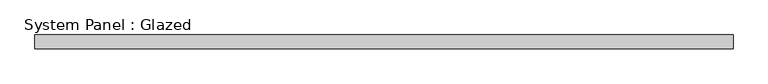
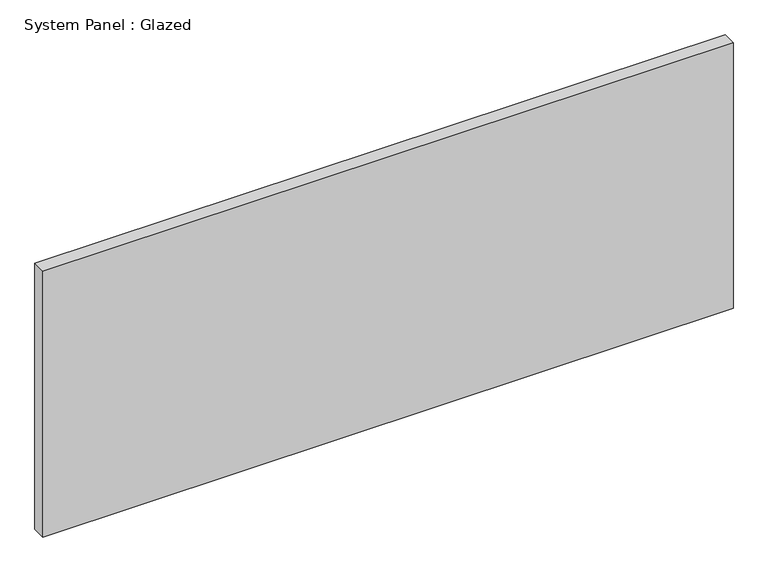
"""IFC4 building model written with IfcOpenShell, lengths in millimetres: plate geometry, System Panel : Glazed."""

from ifc_helpers import new_model, si_unit, origin, origin_with_axes, place, context, project, spatial, polyline, outline, extrude, source, transform, mapped, element, save


def system_panel_glazed_82b35773(model_context):
    return source(origin(), model_context, "Body", "SweptSolid", [
        extrude(outline(polyline([(632.0323546, 19.05), (-632.0323546, 19.05), (-632.0323546, 44.45), (632.0323546, 44.45), (632.0323546, 19.05)])), origin_with_axes(), (0.0, 0.0, 1.0), 514.35),
    ])


if __name__ == "__main__":
    model = new_model("IFC4")
    model_context = context("Model", 3, world=origin())
    ifc_project = project(units=[si_unit("LENGTHUNIT", "METRE", prefix="MILLI")], contexts=[model_context])
    site = spatial("IfcSite", under=ifc_project)
    building = spatial("IfcBuilding", under=site)
    placement = place(None, origin())
    system_panel_glazed_shape = system_panel_glazed_82b35773(model_context)
    element("IfcPlate", 1, ObjectType="System Panel : Glazed", at=placement, inside=building, context=model_context, shape_type="MappedRepresentation", body=[
        mapped(system_panel_glazed_shape, transform((0.0, 0.0, 0.0), x_axis=(1.0, 0.0, 0.0), y_axis=(0.0, 1.0, 0.0), z_axis=(0.0, 0.0, 1.0))),
    ])
    save(model, "model.ifc")

# Revit data of these elements
# Type "System Panel : Glazed"
#   Construction Type Id = "GSP4R"
#   Analytic Construction = "1/8 in Pilkington single glazing"
#   Visual Light Transmittance = 0.9
#   Solar Heat Gain Coefficient = 0.86
#   Heat Transfer Coefficient (U) = 1.18115 BTU/(h·ft²·°F)
#   Define Thermal Properties by = 1
# Element 1 (IfcPlate, "System Panel : Glazed")
#   Materials on its faces: "Glass"
# Materials
#   "Glass": class "Glass", colour RGB 0 128 192, transparency 0.75, Description = "Soda Lime Glass", Cost = 0
